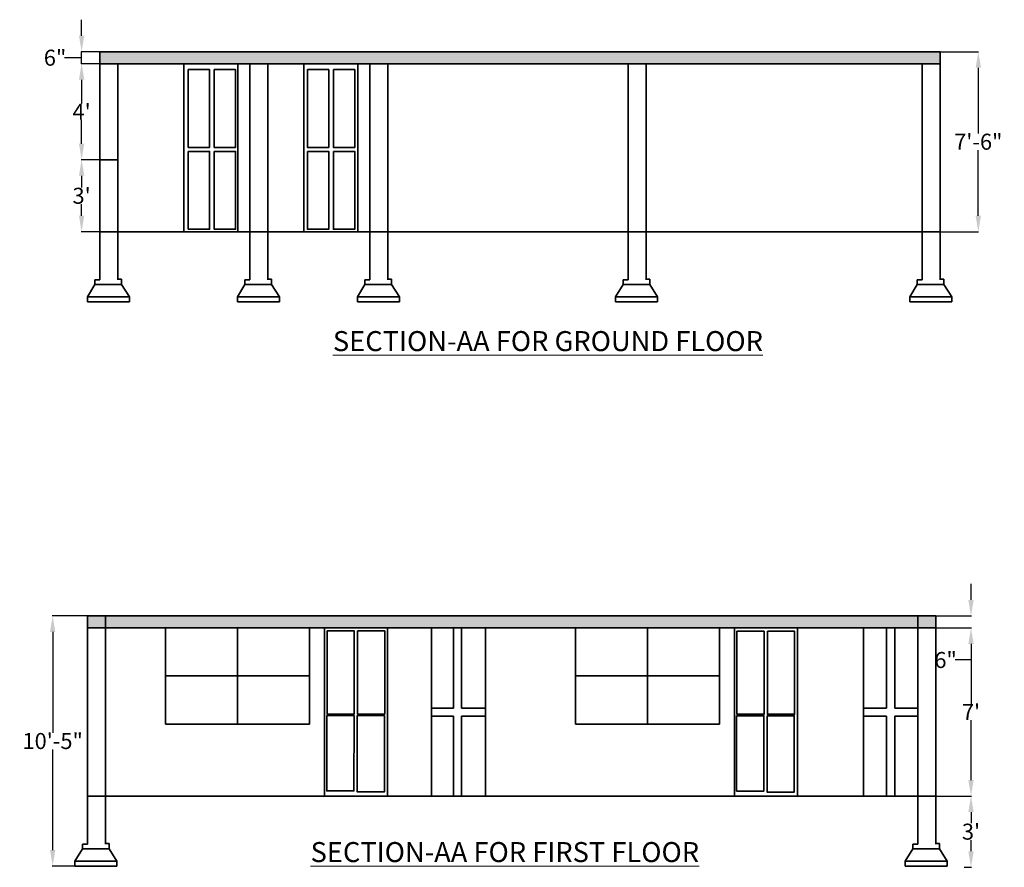
# Model space of a CAD drawing. Units: inches. Extents: x 179 to 2009, y 628 to 2084.
# Tile 2 of 5: x 884 to 1376, y 737 to 1161. Entities that reach past the tile are written whole.
import ezdxf

# ---------------------------------------------------------------- set-up
doc = ezdxf.new("R2010")
doc.units = ezdxf.units.IN
doc.header["$MEASUREMENT"] = 0
for name, color, linetype, lineweight in [('A-ANNO-DIMS', 2, 'Continuous', 18), ('A-ANNO-TEXT', 7, 'Continuous', 18), ('A-SECT', 7, 'Continuous', 35), ('A-SECT-PATT', 8, 'Continuous', 13)]:
    doc.layers.add(name, color=color, linetype=linetype, lineweight=lineweight)
doc.styles.get("Standard").update_dxf_attribs({"font": 'arial.ttf'})
doc.dimstyles.get("Standard").update_dxf_attribs({"dimtxt": 8, "dimasz": 8, "dimexe": 0.18, "dimexo": 0.0625, "dimgap": 0.09, "dimtad": 0, "dimtih": 1, "dimtoh": 1, "dimdec": 0, "dimzin": 0, "dimdsep": 46, "dimlunit": 3, "dimtxsty": 'Standard', "dimcen": 0.09, "dimadec": 0, "dimazin": 0, "dimtfac": 1, "dimtdec": 0, "dimtofl": 0, "dimtmove": 0, "dimatfit": 3, "dimfxl": 1, "dimtolj": 1, "dimtzin": 0, "dimarcsym": 0})

# ---------------------------------------------------------------- blocks, each defined once
blk = doc.blocks.new('*D20')
at = {"layer": 'A-ANNO-DIMS', "color": 0, "lineweight": -2, "transparency": 16777216}
for p, q in [((923.52, 1090.63), (914.3, 1090.63)), ((914.48, 1082.63), (914.48, 1076.81)), ((914.48, 1062.63), (914.48, 1068.45)), ((923.52, 1054.63), (914.3, 1054.63))]:
    blk.add_line(p, q, dxfattribs=at)
at = {"layer": 'A-ANNO-DIMS', "color": 0, "transparency": 16777216}
for points in [[(913.15, 1082.63), (915.82, 1082.63), (914.48, 1090.63)], [(913.15, 1062.63), (915.82, 1062.63), (914.48, 1054.63)]]:
    blk.add_solid(points, dxfattribs=at)
at = {"layer": 'Defpoints', "color": 0, "transparency": 16777216}
for p in [(914.48, 1090.63), (923.58, 1090.63), (923.58, 1054.63)]:
    blk.add_point(p, dxfattribs=at)
at = {"layer": 'A-ANNO-DIMS', "color": 0, "transparency": 16777216, "insert": (914.48, 1072.63), "char_height": 8, "attachment_point": 5}
blk.add_mtext("\\A1;3'", dxfattribs=at)
blk = doc.blocks.new('*D21')
at = {"layer": 'A-ANNO-DIMS', "color": 0, "lineweight": -2, "transparency": 16777216}
for p, q in [((923.52, 1138.63), (914.3, 1138.63)), ((914.48, 1130.63), (914.48, 1118.72)), ((914.48, 1098.63), (914.48, 1110.54)), ((923.52, 1090.63), (914.3, 1090.63))]:
    blk.add_line(p, q, dxfattribs=at)
at = {"layer": 'A-ANNO-DIMS', "color": 0, "transparency": 16777216}
for points in [[(913.15, 1130.63), (915.82, 1130.63), (914.48, 1138.63)], [(913.15, 1098.63), (915.82, 1098.63), (914.48, 1090.63)]]:
    blk.add_solid(points, dxfattribs=at)
at = {"layer": 'Defpoints', "color": 0, "transparency": 16777216}
for p in [(914.48, 1138.63), (923.58, 1138.63), (923.58, 1090.63)]:
    blk.add_point(p, dxfattribs=at)
at = {"layer": 'A-ANNO-DIMS', "color": 0, "transparency": 16777216, "insert": (914.48, 1114.63), "char_height": 8, "attachment_point": 5}
blk.add_mtext("\\A1;4'", dxfattribs=at)
blk = doc.blocks.new('*D22')
at = {"layer": 'A-ANNO-DIMS', "color": 0, "lineweight": -2, "transparency": 16777216}
for p, q in [((914.48, 1152.63), (914.48, 1160.63)), ((923.52, 1144.63), (914.3, 1144.63)), ((914.48, 1138.63), (914.48, 1144.63)), ((906.09, 1141.63), (905.91, 1141.63)), ((914.48, 1141.63), (906.09, 1141.63)), ((923.52, 1138.63), (914.3, 1138.63)), ((914.48, 1130.63), (914.48, 1122.63))]:
    blk.add_line(p, q, dxfattribs=at)
at = {"layer": 'A-ANNO-DIMS', "color": 0, "transparency": 16777216}
for points in [[(913.15, 1152.63), (915.82, 1152.63), (914.48, 1144.63)], [(913.15, 1130.63), (915.82, 1130.63), (914.48, 1138.63)]]:
    blk.add_solid(points, dxfattribs=at)
at = {"layer": 'Defpoints', "color": 0, "transparency": 16777216}
for p in [(914.48, 1144.63), (923.58, 1144.63), (923.58, 1138.63)]:
    blk.add_point(p, dxfattribs=at)
at = {"layer": 'A-ANNO-DIMS', "color": 0, "transparency": 16777216, "insert": (901.2, 1141.63), "char_height": 8, "attachment_point": 5}
blk.add_mtext('\\A1;6"', dxfattribs=at)
blk = doc.blocks.new('*D23')
at = {"layer": 'A-ANNO-DIMS', "color": 0, "lineweight": -2, "transparency": 16777216}
for p, q in [((1343.64, 1144.63), (1362.83, 1144.63)), ((1362.65, 1136.63), (1362.65, 1103.8)), ((1362.65, 1062.63), (1362.65, 1095.45)), ((1343.64, 1054.63), (1362.83, 1054.63))]:
    blk.add_line(p, q, dxfattribs=at)
at = {"layer": 'A-ANNO-DIMS', "color": 0, "transparency": 16777216}
for points in [[(1361.32, 1136.63), (1363.99, 1136.63), (1362.65, 1144.63)], [(1361.32, 1062.63), (1363.99, 1062.63), (1362.65, 1054.63)]]:
    blk.add_solid(points, dxfattribs=at)
at = {"layer": 'Defpoints', "color": 0, "transparency": 16777216}
for p in [(1343.58, 1144.63), (1343.58, 1054.63), (1362.65, 1054.63)]:
    blk.add_point(p, dxfattribs=at)
at = {"layer": 'A-ANNO-DIMS', "color": 0, "transparency": 16777216, "insert": (1362.65, 1099.63), "char_height": 8, "attachment_point": 5}
blk.add_mtext('\\A1;7\'-6"', dxfattribs=at)
blk = doc.blocks.new('*D31')
at = {"layer": 'A-ANNO-DIMS', "color": 0, "lineweight": -2, "transparency": 16777216}
for p, q in [((1359.01, 870.59), (1359.01, 878.59)), ((1341.42, 862.59), (1359.19, 862.59)), ((1341.42, 856.59), (1359.19, 856.59)), ((1359.01, 848.59), (1359.01, 840.59)), ((1359.01, 840.59), (1351.01, 840.59))]:
    blk.add_line(p, q, dxfattribs=at)
at = {"layer": 'A-ANNO-DIMS', "color": 0, "transparency": 16777216}
for points in [[(1357.67, 870.59), (1360.34, 870.59), (1359.01, 862.59)], [(1357.67, 848.59), (1360.34, 848.59), (1359.01, 856.59)]]:
    blk.add_solid(points, dxfattribs=at)
at = {"layer": 'Defpoints', "color": 0, "transparency": 16777216}
for p in [(1341.35, 862.59), (1341.35, 856.59), (1359.01, 856.59)]:
    blk.add_point(p, dxfattribs=at)
at = {"layer": 'A-ANNO-DIMS', "color": 0, "transparency": 16777216, "insert": (1346.3, 840.59), "char_height": 8, "attachment_point": 5}
blk.add_mtext('\\A1;6"', dxfattribs=at)
blk = doc.blocks.new('*D32')
at = {"layer": 'A-ANNO-DIMS', "color": 0, "lineweight": -2, "transparency": 16777216}
for p, q in [((1341.42, 856.59), (1359.19, 856.59)), ((1359.01, 848.59), (1359.01, 818.68)), ((1359.01, 780.59), (1359.01, 810.5)), ((1341.42, 772.59), (1359.19, 772.59))]:
    blk.add_line(p, q, dxfattribs=at)
at = {"layer": 'A-ANNO-DIMS', "color": 0, "transparency": 16777216}
for points in [[(1357.67, 848.59), (1360.34, 848.59), (1359.01, 856.59)], [(1357.67, 780.59), (1360.34, 780.59), (1359.01, 772.59)]]:
    blk.add_solid(points, dxfattribs=at)
at = {"layer": 'Defpoints', "color": 0, "transparency": 16777216}
for p in [(1341.35, 856.59), (1341.35, 772.59), (1359.01, 772.59)]:
    blk.add_point(p, dxfattribs=at)
at = {"layer": 'A-ANNO-DIMS', "color": 0, "transparency": 16777216, "insert": (1359.01, 814.59), "char_height": 8, "attachment_point": 5}
blk.add_mtext("\\A1;7'", dxfattribs=at)
blk = doc.blocks.new('*D33')
at = {"layer": 'A-ANNO-DIMS', "color": 0, "lineweight": -2, "transparency": 16777216}
for p, q in [((1341.42, 772.59), (1359.19, 772.59)), ((1359.01, 764.59), (1359.01, 758.95)), ((1359.01, 744.97), (1359.01, 750.6)), ((1355.61, 736.97), (1359.19, 736.97))]:
    blk.add_line(p, q, dxfattribs=at)
at = {"layer": 'A-ANNO-DIMS', "color": 0, "transparency": 16777216}
for points in [[(1357.67, 764.59), (1360.34, 764.59), (1359.01, 772.59)], [(1357.67, 744.97), (1360.34, 744.97), (1359.01, 736.97)]]:
    blk.add_solid(points, dxfattribs=at)
at = {"layer": 'Defpoints', "color": 0, "transparency": 16777216}
for p in [(1341.35, 772.59), (1355.54, 736.97), (1359.01, 736.97)]:
    blk.add_point(p, dxfattribs=at)
at = {"layer": 'A-ANNO-DIMS', "color": 0, "transparency": 16777216, "insert": (1359.01, 754.78), "char_height": 8, "attachment_point": 5}
blk.add_mtext("\\A1;3'", dxfattribs=at)
blk = doc.blocks.new('*D34')
at = {"layer": 'A-ANNO-DIMS', "color": 0, "lineweight": -2, "transparency": 16777216}
for p, q in [((917.29, 862.59), (899.85, 862.59)), ((900.03, 854.59), (900.03, 804.26)), ((900.03, 745.59), (900.03, 795.92)), ((917.29, 737.59), (899.85, 737.59))]:
    blk.add_line(p, q, dxfattribs=at)
at = {"layer": 'A-ANNO-DIMS', "color": 0, "transparency": 16777216}
for points in [[(898.69, 854.59), (901.36, 854.59), (900.03, 862.59)], [(898.69, 745.59), (901.36, 745.59), (900.03, 737.59)]]:
    blk.add_solid(points, dxfattribs=at)
at = {"layer": 'Defpoints', "color": 0, "transparency": 16777216}
for p in [(917.35, 862.59), (900.03, 737.59), (917.35, 737.59)]:
    blk.add_point(p, dxfattribs=at)
at = {"layer": 'A-ANNO-DIMS', "color": 0, "transparency": 16777216, "insert": (900.03, 800.09), "char_height": 8, "attachment_point": 5}
blk.add_mtext('\\A1;10\'-5"', dxfattribs=at)

msp = doc.modelspace()

# ---------------------------------------------------------------- hatches: boundary and pattern name
at = {"layer": 'A-SECT-PATT'}
h = msp.add_hatch(dxfattribs=at)
h.set_pattern_fill('AR-CONC', color=256)
h.set_pattern_definition([(50, (0, 0), (7.172602, -0.627521), [0.75, -8.25]), (355, (0, 0), (-1.387513, 7.52192), [0.6, -6.6]), (100.45144, (0.598, -0.052), (5.785088, 6.8944), [0.637402, -7.01142]), (46.1842, (0, 2), (10.672413, -1.655193), [1.125, -12.375]), (96.63564, (0.889, 1.862), (9.34662, 9.741186), [0.956103, -10.51714]), (351.18416, (0, 2), (9.34662, 9.741186), [0.9, -9.9]), (21, (1, 1.5), (5.96907, -4.026189), [0.75, -8.25]), (326, (1, 1.5), (2.433153, 7.2515), [0.6, -6.6]), (71.45144, (1.4974, 1.1645), (8.402224, 3.225312), [0.637402, -7.01142]), (37.5, (0, 0), (0.1215986, 3.3289385), [0, -6.52, 0, -6.7, 0, -6.625]), (7.5, (0, 0), (2.6306954, 3.944117), [0, -3.82, 0, -6.37, 0, -2.525]), (327.5, (-2.23, 0), (5.3382244, -0.2255487), [0, -2.5, 0, -7.8, 0, -10.35]), (317.5, (-3.23, 0), (5.831862, 1.00105), [0, -3.25, 0, -5.18, 0, -7.35])])
h.paths.add_polyline_path([(1332.35, 862.59), (926.35, 862.59), (926.35, 856.59), (1332.35, 856.59)])
h.paths.add_polyline_path([(1341.35, 862.59), (1332.35, 862.59), (1332.35, 856.59), (1341.35, 856.59)])
h.paths.add_polyline_path([(926.35, 862.59), (917.35, 862.59), (917.35, 856.59), (926.35, 856.59)])
h.paths.add_polyline_path([(1343.58, 1144.63), (923.58, 1144.63), (923.58, 1138.63), (1343.58, 1138.63)])

# ---------------------------------------------------------------- linework, layer by layer
at = {"layer": 'A-SECT'}
for p, q in [((923.58, 1054.63), (923.58, 1144.63)), ((923.58, 1144.63), (1343.58, 1144.63)), ((1343.58, 1054.63), (1343.58, 1144.63)), ((923.58, 1138.63), (1343.58, 1138.63)), ((932.58, 1054.63), (932.58, 1138.63)), ((965.5, 1054.63), (965.5, 1138.63)), ((992.5, 1054.63), (992.5, 1138.63)), ((998.58, 1054.63), (998.58, 1138.63)), ((1007.58, 1054.63), (1007.58, 1138.63)), ((1025.58, 1054.63), (1025.58, 1138.63)), ((1052.58, 1054.63), (1052.58, 1138.63)), ((1058.58, 1054.63), (1058.58, 1138.63)), ((1067.58, 1054.63), (1067.58, 1138.63)), ((1187.58, 1054.63), (1187.58, 1138.63)), ((1196.58, 1054.63), (1196.58, 1138.63)), ((1334.58, 1054.63), (1334.58, 1138.63)), ((923.58, 1090.63), (932.58, 1090.63)), ((923.58, 1054.63), (1343.58, 1054.63)), ((923.58, 1054.63), (923.58, 1030.63)), ((932.58, 1054.63), (932.58, 1030.63)), ((998.58, 1054.63), (998.58, 1030.63)), ((1007.58, 1054.63), (1007.58, 1030.63)), ((1058.58, 1054.63), (1058.58, 1030.63)), ((1067.58, 1054.63), (1067.58, 1030.63)), ((1187.58, 1054.63), (1187.58, 1030.63)), ((1196.58, 1054.63), (1196.58, 1030.63)), ((1334.58, 1054.63), (1334.58, 1030.63)), ((1343.58, 1054.63), (1343.58, 1030.63)), ((923.58, 1030.63), (921.1, 1030.63)), ((921.1, 1030.63), (921.1, 1028.2)), ((934.41, 1030.91), (932.58, 1030.91)), ((934.41, 1028.2), (934.41, 1030.91)), ((998.58, 1030.63), (996.1, 1030.63)), ((996.1, 1030.63), (996.1, 1028.2)), ((1009.41, 1030.91), (1007.58, 1030.91)), ((1009.41, 1028.2), (1009.41, 1030.91)), ((1058.58, 1030.63), (1056.1, 1030.63)), ((1056.1, 1030.63), (1056.1, 1028.2)), ((1069.41, 1030.91), (1067.58, 1030.91)), ((1069.41, 1028.2), (1069.41, 1030.91)), ((1187.58, 1030.63), (1185.1, 1030.63)), ((1185.1, 1030.63), (1185.1, 1028.2)), ((1198.41, 1030.91), (1196.58, 1030.91)), ((1198.41, 1028.2), (1198.41, 1030.91)), ((1334.58, 1030.63), (1332.1, 1030.63)), ((1332.1, 1030.63), (1332.1, 1028.2)), ((1345.41, 1030.91), (1343.58, 1030.91)), ((1345.41, 1028.2), (1345.41, 1030.91)), ((921.1, 1028.2), (917.37, 1022.14)), ((921.1, 1028.2), (934.41, 1028.2)), ((938.36, 1022.14), (934.41, 1028.2)), ((996.1, 1028.2), (992.37, 1022.14)), ((996.1, 1028.2), (1009.41, 1028.2)), ((1013.36, 1022.14), (1009.41, 1028.2)), ((1056.1, 1028.2), (1052.37, 1022.14)), ((1056.1, 1028.2), (1069.41, 1028.2)), ((1073.36, 1022.14), (1069.41, 1028.2)), ((1185.1, 1028.2), (1181.37, 1022.14)), ((1185.1, 1028.2), (1198.41, 1028.2)), ((1202.36, 1022.14), (1198.41, 1028.2)), ((1332.1, 1028.2), (1328.37, 1022.14)), ((1332.1, 1028.2), (1345.41, 1028.2)), ((1349.36, 1022.14), (1345.41, 1028.2)), ((917.37, 1022.14), (938.36, 1022.14)), ((917.37, 1022.14), (917.37, 1019.63)), ((917.37, 1019.63), (938.35, 1019.63)), ((938.35, 1019.63), (938.35, 1022.14)), ((992.37, 1022.14), (1013.36, 1022.14)), ((992.37, 1022.14), (992.37, 1019.63)), ((992.37, 1019.63), (1013.35, 1019.63)), ((1013.35, 1019.63), (1013.35, 1022.14)), ((1052.37, 1022.14), (1073.36, 1022.14)), ((1052.37, 1022.14), (1052.37, 1019.63)), ((1052.37, 1019.63), (1073.35, 1019.63)), ((1073.35, 1019.63), (1073.35, 1022.14)), ((1181.37, 1022.14), (1202.36, 1022.14)), ((1181.37, 1022.14), (1181.37, 1019.63)), ((1181.37, 1019.63), (1202.35, 1019.63)), ((1202.35, 1019.63), (1202.35, 1022.14)), ((1328.37, 1022.14), (1349.36, 1022.14)), ((1328.37, 1022.14), (1328.37, 1019.63)), ((1328.37, 1019.63), (1349.35, 1019.63)), ((1349.35, 1019.63), (1349.35, 1022.14)), ((917.35, 862.59), (1341.35, 862.59)), ((917.35, 772.59), (917.35, 862.59)), ((926.35, 772.59), (926.35, 862.59)), ((1332.35, 772.59), (1332.35, 862.59)), ((1341.35, 772.59), (1341.35, 862.59)), ((917.35, 856.59), (1341.35, 856.59)), ((956.35, 808.59), (956.35, 856.59)), ((992.35, 808.59), (992.35, 856.59)), ((1028.35, 808.59), (1028.35, 856.59)), ((1035.85, 772.59), (1035.85, 856.59)), ((1067.35, 772.59), (1067.35, 856.59)), ((1089.35, 772.59), (1089.35, 856.59)), ((1100.42, 816.59), (1100.42, 856.59)), ((1104.42, 816.59), (1104.42, 856.59)), ((1116.35, 772.59), (1116.35, 856.59)), ((1161.35, 808.59), (1161.35, 856.59)), ((1197.35, 808.59), (1197.35, 856.59)), ((1233.35, 808.59), (1233.35, 856.59)), ((1240.85, 772.59), (1240.85, 856.59)), ((1272.35, 772.59), (1272.35, 856.59)), ((1305.35, 772.59), (1305.35, 856.59)), ((1316.85, 856.59), (1316.85, 816.59)), ((1320.85, 856.59), (1320.85, 816.59)), ((956.35, 832.59), (1028.35, 832.59)), ((1161.35, 832.59), (1233.35, 832.59)), ((1089.35, 816.59), (1100.42, 816.59)), ((1089.35, 812.59), (1100.42, 812.59)), ((1100.42, 772.59), (1100.42, 812.59)), ((1104.42, 816.59), (1116.35, 816.59)), ((1104.42, 812.59), (1116.35, 812.59)), ((1104.42, 772.59), (1104.42, 812.59)), ((1305.35, 816.59), (1316.85, 816.59)), ((1305.35, 812.59), (1316.85, 812.59)), ((1316.85, 812.59), (1316.85, 772.59)), ((1320.85, 816.59), (1332.35, 816.59)), ((1320.85, 812.59), (1320.85, 772.59)), ((1320.85, 812.59), (1332.35, 812.59)), ((956.35, 808.59), (1028.35, 808.59)), ((1161.35, 808.59), (1233.35, 808.59)), ((917.35, 772.59), (1341.35, 772.59)), ((917.35, 772.59), (917.35, 748.59)), ((926.35, 772.59), (926.35, 748.59)), ((1332.35, 772.59), (1332.35, 748.59)), ((1341.35, 772.59), (1341.35, 748.59)), ((917.35, 748.59), (914.87, 748.59)), ((914.87, 748.59), (914.87, 746.16)), ((928.18, 748.87), (926.35, 748.87)), ((928.18, 746.16), (928.18, 748.87)), ((1332.35, 748.59), (1329.87, 748.59)), ((1329.87, 748.59), (1329.87, 746.16)), ((1343.18, 748.87), (1341.35, 748.87)), ((1343.18, 746.16), (1343.18, 748.87)), ((914.87, 746.16), (911.15, 740.1)), ((914.87, 746.16), (928.18, 746.16)), ((932.13, 740.1), (928.18, 746.16)), ((1329.87, 746.16), (1326.15, 740.1)), ((1329.87, 746.16), (1343.18, 746.16)), ((1347.13, 740.1), (1343.18, 746.16)), ((911.15, 740.1), (932.13, 740.1)), ((911.15, 740.1), (911.15, 737.59)), ((932.12, 737.59), (932.12, 740.1)), ((1326.15, 740.1), (1347.13, 740.1)), ((1326.15, 740.1), (1326.15, 737.59)), ((1347.12, 737.59), (1347.12, 740.1)), ((911.15, 737.59), (932.12, 737.59)), ((1326.15, 737.59), (1347.12, 737.59))]:
    msp.add_line(p, q, dxfattribs=at)
for points in [[(967.79, 1135.73), (978.47, 1135.73), (978.47, 1096.82), (967.79, 1096.82)], [(980.8, 1135.73), (991.48, 1135.73), (991.48, 1096.82), (980.8, 1096.82)], [(1027.31, 1135.73), (1037.99, 1135.73), (1037.99, 1096.82), (1027.31, 1096.82)], [(1040.32, 1135.73), (1051, 1135.73), (1051, 1096.82), (1040.32, 1096.82)], [(967.79, 1094.83), (978.47, 1094.83), (978.47, 1055.92), (967.79, 1055.92)], [(980.8, 1094.83), (991.48, 1094.83), (991.48, 1055.92), (980.8, 1055.92)], [(1027.31, 1094.83), (1037.99, 1094.83), (1037.99, 1055.92), (1027.31, 1055.92)], [(1040.32, 1094.83), (1051, 1094.83), (1051, 1055.92), (1040.32, 1055.92)], [(1037.17, 855.1), (1050.75, 855.1), (1050.75, 813.57), (1037.17, 813.57)], [(1052.41, 855.1), (1065.99, 855.1), (1065.99, 813.57), (1052.41, 813.57)], [(1242.01, 854.98), (1255.59, 854.98), (1255.59, 813.45), (1242.01, 813.45)], [(1257.24, 854.98), (1270.82, 854.98), (1270.82, 813.45), (1257.24, 813.45)], [(1037.05, 812.84), (1050.63, 812.84), (1050.59, 775.15), (1037.01, 775.15)], [(1052.28, 812.84), (1065.86, 812.84), (1065.8, 774.65), (1052.22, 774.65)], [(1241.88, 812.72), (1255.46, 812.72), (1255.43, 775.03), (1241.84, 775.03)], [(1257.12, 812.72), (1270.7, 812.72), (1270.64, 774.53), (1257.06, 774.53)]]:
    msp.add_lwpolyline(points, close=True, dxfattribs=at)

# ---------------------------------------------------------------- texts
at = {"layer": 'A-ANNO-TEXT', "char_height": 10, "attachment_point": 1}
for s, insert in [('{\\fArial|b1|i0|c0|p34;\\LSECTION-AA FOR GROUND FLOOR}', (1040.08, 1004.98)), ('{\\fArial|b1|i0|c0|p34;\\LSECTION-AA FOR FIRST FLOOR}', (1028.93, 749.58))]:
    msp.add_mtext_dynamic_manual_height_columns(s, width=224.9889, gutter_width=1, heights=[0], dxfattribs=dict(at, insert=insert))

# ---------------------------------------------------------------- dimensions: what is measured, and where the dimension line sits
at = {"layer": 'A-ANNO-DIMS'}
for base, p1, p2, override, picture, middle in [((914.48, 1144.63), (923.58, 1138.63), (923.58, 1144.63), {"dimclrd": 0, "dimclre": 0, "dimclrt": 0, "dimtmove": 1}, '*D22', (905.82, 1141.63)), ((1362.65, 1054.63), (1343.58, 1144.63), (1343.58, 1054.63), {"dimclrd": 0, "dimclre": 0, "dimclrt": 0}, '*D23', (1362.65, 1099.63)), ((914.48, 1138.63), (923.58, 1090.63), (923.58, 1138.63), {"dimclrd": 0, "dimclre": 0, "dimclrt": 0, "dimtmove": 1}, '*D21', (914.48, 1114.63)), ((914.48, 1090.63), (923.58, 1054.63), (923.58, 1090.63), {"dimclrd": 0, "dimclre": 0, "dimclrt": 0}, '*D20', (914.48, 1072.63)), ((1359.01, 856.59), (1341.35, 862.59), (1341.35, 856.59), {"dimclrd": 0, "dimclre": 0, "dimclrt": 0}, '*D31', (1346.3, 840.59)), ((900.03, 737.59), (917.35, 862.59), (917.35, 737.59), {"dimclrd": 0, "dimclre": 0, "dimclrt": 0}, '*D34', (900.03, 800.09)), ((1359.01, 772.59), (1341.35, 856.59), (1341.35, 772.59), {"dimclrd": 0, "dimclre": 0, "dimclrt": 0, "dimtmove": 1}, '*D32', (1359.01, 814.59)), ((1359.01, 736.97), (1341.35, 772.59), (1355.54, 736.97), {"dimclrd": 0, "dimclre": 0, "dimclrt": 0, "dimtmove": 1}, '*D33', (1359.01, 754.78))]:
    dim = msp.add_linear_dim(base=base, p1=p1, p2=p2, angle=90, dimstyle='Standard', override=override, dxfattribs=at)
    dim.commit()
    dim.dimension.update_dxf_attribs({"geometry": picture, "text_midpoint": middle})

doc.saveas('drawing.dxf')
